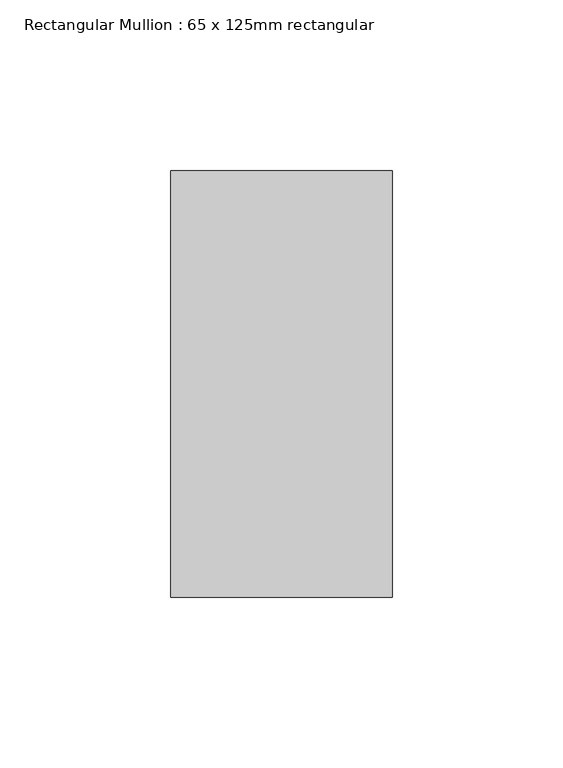
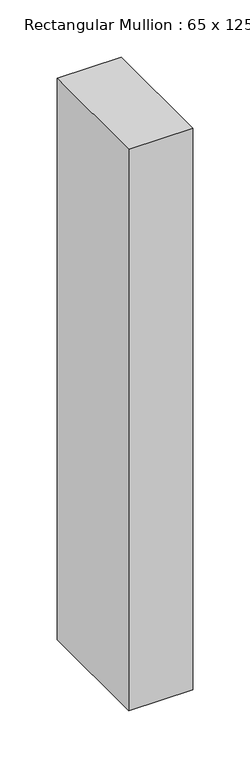
"""IFC4 building model written with IfcOpenShell, lengths in millimetres: member geometry, Rectangular Mullion : 65 x 125mm rectangular."""

from ifc_helpers import new_model, si_unit, frame, origin, place, context, project, spatial, polyline, outline, extrude, source, transform, mapped, element, save


def rectangular_mullion_65_x_125mm_rectangular_1b222a86(model_context):
    return source(origin(), model_context, "Body", "SweptSolid", [
        extrude(outline(polyline([(32.5, 62.5), (32.5, -62.5), (-32.5, -62.5), (-32.5, 62.5), (32.5, 62.5)])), frame((0.0, 0.0, -600.0), z_axis=(0.0, 0.0, 1.0), x_axis=(1.0, 0.0, 0.0)), (0.0, 0.0, 1.0), 600.0),
    ])


if __name__ == "__main__":
    model = new_model("IFC4")
    model_context = context("Model", 3, world=origin())
    ifc_project = project(units=[si_unit("LENGTHUNIT", "METRE", prefix="MILLI")], contexts=[model_context])
    site = spatial("IfcSite", under=ifc_project)
    building = spatial("IfcBuilding", under=site)
    placement = place(None, origin())
    rectangular_mullion_65_x_125mm_rectangular_shape = rectangular_mullion_65_x_125mm_rectangular_1b222a86(model_context)
    element("IfcMember", 1, ObjectType="Rectangular Mullion : 65 x 125mm rectangular", at=placement, inside=building, context=model_context, shape_type="MappedRepresentation", body=[
        mapped(rectangular_mullion_65_x_125mm_rectangular_shape, transform((0.0, 0.0, 0.0), x_axis=(1.0, 0.0, 0.0), y_axis=(0.0, 1.0, 0.0), z_axis=(0.0, 0.0, 1.0))),
    ])
    save(model, "model.ifc")

# Revit data of these elements
# Type "Rectangular Mullion : 65 x 125mm rectangular"
#   built-in parameter 1007304 = 0.410105 (stored number, unit not read)
#   built-in parameter 1007301 = 0.106627 (stored number, unit not read)
#   built-in parameter 1007300 = 0.106627 (stored number, unit not read)
# Element 1 (IfcMember, "Rectangular Mullion : 65 x 125mm rectangular")
#   Materials on its faces: "Aluminum"
# Materials
#   "Aluminum": class "Metal", colour RGB 244 245 246, transparency 0, Description = "Aluminum 6061", Cost = 0
